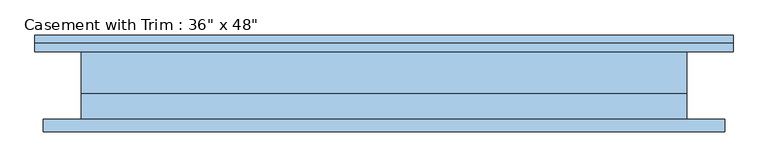
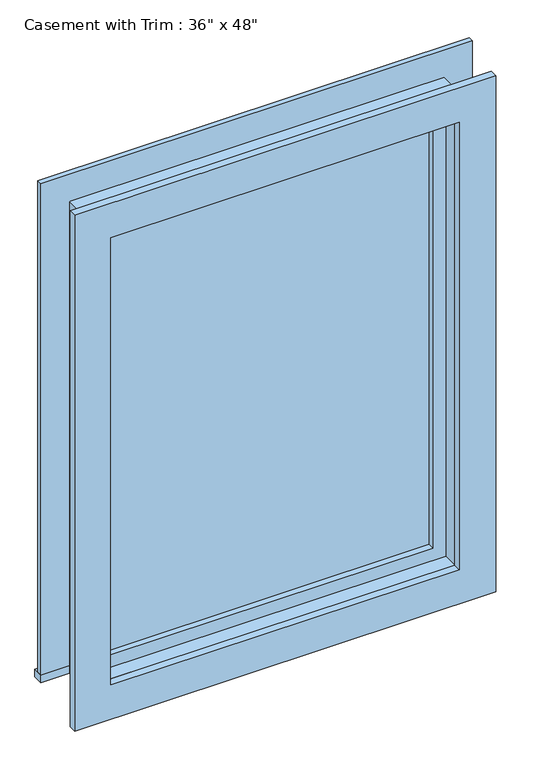
"""IFC4 building model written with IfcOpenShell, lengths in millimetres: window geometry."""

from ifc_helpers import new_model, si_unit, frame, origin, place, context, project, spatial, polyline, outline, extrude, source, transform, mapped, element, save


def window_2df9a94c(model_context):
    return source(origin(), model_context, "Body", "SweptSolid", [
        extrude(outline(polyline([(-527.05, 76.2), (527.05, 76.2), (527.05, 50.8), (-527.05, 50.8), (-527.05, 76.2)])), frame((0.0, 0.0, 914.4), z_axis=(0.0, 0.0, 1.0), x_axis=(1.0, 0.0, 0.0)), (0.0, 0.0, 1.0), 19.05),
        extrude(outline(polyline([(2114.55, -438.15), (2114.55, 438.15), (933.45, 438.15), (933.45, 527.05), (2203.45, 527.05), (2203.45, -527.05), (933.45, -527.05), (933.45, -438.15), (2114.55, -438.15)])), frame((0.0, 50.8, 0.0), z_axis=(0.0, 1.0, 0.0), x_axis=(0.0, 0.0, 1.0)), (0.0, 0.0, 1.0), 12.7),
        extrude(outline(polyline([(2190.75, 514.35), (2190.75, -514.35), (857.25, -514.35), (857.25, 514.35), (2190.75, 514.35)]), holes=[polyline([(2101.85, 425.45), (946.15, 425.45), (946.15, -425.45), (2101.85, -425.45), (2101.85, 425.45)])]), frame((0.0, -69.85, 0.0), z_axis=(0.0, 1.0, 0.0), x_axis=(0.0, 0.0, 1.0)), (0.0, 0.0, 1.0), 19.05),
        extrude(outline(polyline([(393.7, 3.175), (-393.7, 3.175), (-393.7, 15.875), (393.7, 15.875), (393.7, 3.175)])), frame((0.0, 0.0, 977.9), z_axis=(0.0, 0.0, 1.0), x_axis=(1.0, 0.0, 0.0)), (0.0, 0.0, 1.0), 1092.2),
        extrude(outline(polyline([(2114.55, -438.15), (933.45, -438.15), (933.45, 438.15), (2114.55, 438.15), (2114.55, -438.15)]), holes=[polyline([(2070.1, -393.7), (2070.1, 393.7), (977.9, 393.7), (977.9, -393.7), (2070.1, -393.7)])]), frame((0.0, -12.7, 0.0), z_axis=(0.0, 1.0, 0.0), x_axis=(0.0, 0.0, 1.0)), (0.0, 0.0, 1.0), 44.45),
        extrude(outline(polyline([(2133.6, -457.2), (914.4, -457.2), (914.4, 457.2), (2133.6, 457.2), (2133.6, -457.2)]), holes=[polyline([(2101.85, -425.45), (2101.85, 425.45), (946.15, 425.45), (946.15, -425.45), (2101.85, -425.45)])]), frame((0.0, -50.8, 0.0), z_axis=(0.0, 1.0, 0.0), x_axis=(0.0, 0.0, 1.0)), (0.0, 0.0, 1.0), 38.1),
        extrude(outline(polyline([(2133.6, 457.2), (2133.6, -457.2), (914.4, -457.2), (914.4, 457.2), (2133.6, 457.2)]), holes=[polyline([(2114.55, 438.15), (933.45, 438.15), (933.45, -438.15), (2114.55, -438.15), (2114.55, 438.15)])]), frame((0.0, -12.7, 0.0), z_axis=(0.0, 1.0, 0.0), x_axis=(0.0, 0.0, 1.0)), (0.0, 0.0, 1.0), 63.5),
    ])


if __name__ == "__main__":
    model = new_model("IFC4")
    model_context = context("Model", 3, world=origin())
    ifc_project = project(units=[si_unit("LENGTHUNIT", "METRE", prefix="MILLI")], contexts=[model_context])
    site = spatial("IfcSite", under=ifc_project)
    building = spatial("IfcBuilding", under=site)
    placement = place(None, origin())
    window_shape = window_2df9a94c(model_context)
    element("IfcWindow", 1, ObjectType="Casement with Trim : 36\" x 48\"", at=placement, inside=building, context=model_context, shape_type="MappedRepresentation", body=[
        mapped(window_shape, transform((0.0, 0.0, 0.0), x_axis=(1.0, 0.0, 0.0), y_axis=(0.0, 1.0, 0.0), z_axis=(0.0, 0.0, 1.0))),
    ])
    save(model, "model.ifc")

# Revit data of these elements
# Type "Casement with Trim : 36\" x 48\""
#   Type Mark = "10"
#   Construction Type Id = "GSP4R"
#   Assembly Code = "B2020100"
#   Analytic Construction = "1/8 in Pilkington single glazing"
#   Visual Light Transmittance = 0.9
#   Solar Heat Gain Coefficient = 0.78
#   Heat Transfer Coefficient (U) = 0.6496 BTU/(h·ft²·°F)
#   Height = 4' - 0"
#   Default Sill Height = 3' - 0"
#   Trim Projection - Ext. = 0' - 0 1/2"
#   Trim Projection - Int. = 0' - 0 3/4"
#   Trim Width - Exterior = 0' - 3 1/2"
#   Trim Width - Interior = 0' - 3 1/2"
#   Width = 3' - 0"
#   Window Inset = 0' - 0 3/4"
#   Define Thermal Properties by = 1
#   Glass Pane Material = Glass
#   Sash Material = Sash
#   Trim Exterior Material = Trim
#   Trim Interior Material = Trim
#   Wall Closure = (empty or 0)
# Element 1 (IfcWindow, "Casement with Trim : 36\" x 48\"")
#   Materials on its faces: "Sash", "Trim", "Glass"
# Materials
#   "Glass": class "Glass", colour RGB 0 128 192, transparency 0.75, Description = "Soda Lime Glass", Cost = 0
#   "Sash": class "Wood", colour RGB 224 178 126, transparency 0
#   "Trim": class "Wood", colour RGB 224 178 126, transparency 0
